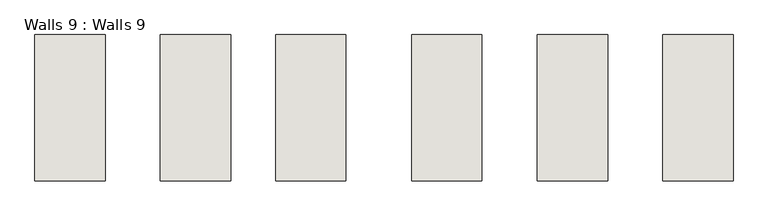
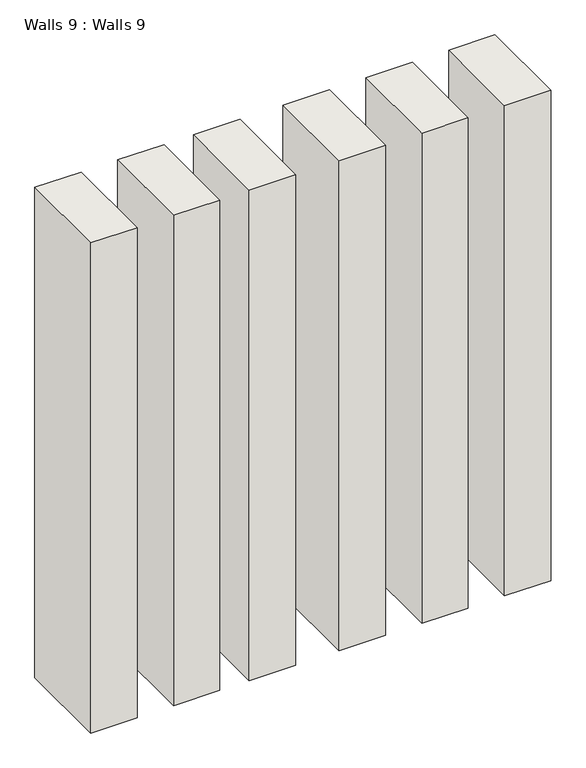
"""IFC4 building model written with IfcOpenShell, lengths in millimetres: wall geometry, Walls 9 : Walls 9."""

from ifc_helpers import new_model, si_unit, frame, origin, place, context, project, spatial, polyline, outline, extrude, source, transform, mapped, element, save


def walls_9_walls_9_54edce94(model_context):
    return source(origin(), model_context, "Body", "SweptSolid", [
        extrude(outline(polyline([(-9850.5527129, -4005.8259649), (-10021.1728698, -4005.8259649), (-10021.1728698, -3650.2259649), (-9850.5527129, -3650.2259649), (-9850.5527129, -4005.8259649)])), frame((0.0, 0.0, 7830.2560163), z_axis=(0.0, 0.0, 1.0), x_axis=(1.0, 0.0, 0.0)), (0.0, 0.0, 1.0), 1906.9611818),
        extrude(outline(polyline([(-9545.7527129, -4005.8259649), (-9716.3728698, -4005.8259649), (-9716.3728698, -3650.2259649), (-9545.7527129, -3650.2259649), (-9545.7527129, -4005.8259649)])), frame((0.0, 0.0, 7830.2560163), z_axis=(0.0, 0.0, 1.0), x_axis=(1.0, 0.0, 0.0)), (0.0, 0.0, 1.0), 1906.9611818),
        extrude(outline(polyline([(-9266.3527129, -4005.8259649), (-9436.9728698, -4005.8259649), (-9436.9728698, -3650.2259649), (-9266.3527129, -3650.2259649), (-9266.3527129, -4005.8259649)])), frame((0.0, 0.0, 7830.2560163), z_axis=(0.0, 0.0, 1.0), x_axis=(1.0, 0.0, 0.0)), (0.0, 0.0, 1.0), 1906.9611818),
        extrude(outline(polyline([(-8936.1527129, -4005.8259649), (-9106.7728698, -4005.8259649), (-9106.7728698, -3650.2259649), (-8936.1527129, -3650.2259649), (-8936.1527129, -4005.8259649)])), frame((0.0, 0.0, 7830.2560163), z_axis=(0.0, 0.0, 1.0), x_axis=(1.0, 0.0, 0.0)), (0.0, 0.0, 1.0), 1906.9611818),
        extrude(outline(polyline([(-8631.3527129, -4005.8259649), (-8801.9728698, -4005.8259649), (-8801.9728698, -3650.2259649), (-8631.3527129, -3650.2259649), (-8631.3527129, -4005.8259649)])), frame((0.0, 0.0, 7830.2560163), z_axis=(0.0, 0.0, 1.0), x_axis=(1.0, 0.0, 0.0)), (0.0, 0.0, 1.0), 1906.9611818),
        extrude(outline(polyline([(-8326.5527129, -4005.8259649), (-8497.1728698, -4005.8259649), (-8497.1728698, -3650.2259649), (-8326.5527129, -3650.2259649), (-8326.5527129, -4005.8259649)])), frame((0.0, 0.0, 7830.2560163), z_axis=(0.0, 0.0, 1.0), x_axis=(1.0, 0.0, 0.0)), (0.0, 0.0, 1.0), 1906.9611818),
    ])


if __name__ == "__main__":
    model = new_model("IFC4")
    model_context = context("Model", 3, world=origin())
    ifc_project = project(units=[si_unit("LENGTHUNIT", "METRE", prefix="MILLI")], contexts=[model_context])
    site = spatial("IfcSite", under=ifc_project)
    building = spatial("IfcBuilding", under=site)
    placement = place(None, origin())
    walls_9_walls_9_shape = walls_9_walls_9_54edce94(model_context)
    element("IfcWall", 1, ObjectType="Walls 9 : Walls 9", at=placement, inside=building, context=model_context, shape_type="MappedRepresentation", body=[
        mapped(walls_9_walls_9_shape, transform((0.0, 0.0, 0.0), x_axis=(1.0, 0.0, 0.0), y_axis=(0.0, 1.0, 0.0), z_axis=(0.0, 0.0, 1.0))),
    ])
    save(model, "model.ifc")

# Revit data of these elements
# Element 1 (IfcWall, "Walls 9 : Walls 9")
#   Materials on its faces: "Default Wall"
# Materials
#   "Default Wall": colour RGB 128 128 128, transparency 0
